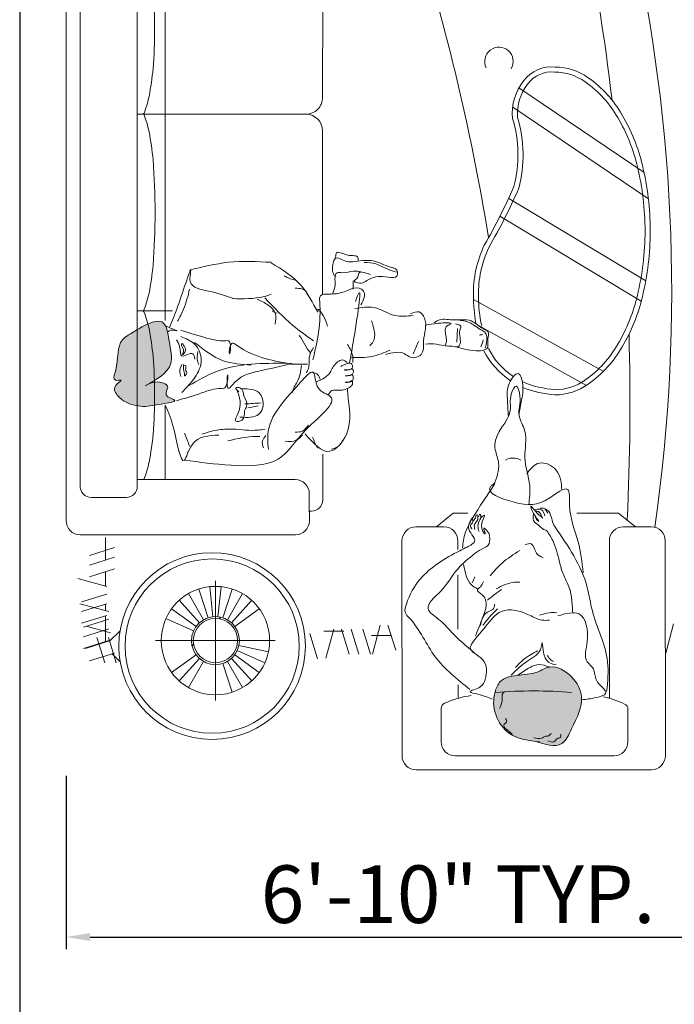
# Model space of a CAD drawing. Units: millimetres. Extents: x 20768 to 23556, y 50760 to 52704.
# Tile 10 of 36: x 20908 to 20976, y 51904 to 52007. Entities that reach past the tile are written whole.
import ezdxf

# ---------------------------------------------------------------- set-up
doc = ezdxf.new("R2010")
doc.units = ezdxf.units.MM
doc.layers.add('A-FURN', color=8, linetype='Continuous', lineweight=18)
doc.layers.add('S-ANNO-DIMS', color=2, linetype='Continuous', lineweight=18)
doc.styles.get("Standard").update_dxf_attribs({"font": 'arial.ttf'})
doc.dimstyles.new('ISO-25', dxfattribs={"dimtxt": 6, "dimasz": 2.5, "dimexe": 1.25, "dimexo": 0.625, "dimtad": 1, "dimdec": 0, "dimlunit": 3, "dimtxsty": 'Standard', "dimcen": 2.5, "dimadec": 0, "dimazin": 0, "dimtfac": 1, "dimtdec": 0, "dimtmove": 0, "dimatfit": 3, "dimfxl": 1, "dimarcsym": 0})

# ---------------------------------------------------------------- blocks, each defined once
blk = doc.blocks.new('A$C32DD204E')
at = {"ltscale": 3}
h = blk.add_hatch(color=256, dxfattribs=at)
edge = h.paths.add_edge_path()
edge.add_spline(control_points=[(248.5, 1171), (279.6, 1188.5), (331.5, 1220.4), (312.1, 1296.2), (303.9, 1374.7), (243.4, 1354.4), (209.2, 1331.9), (147.9, 1299.6), (163.4, 1244.6), (138.6, 1178), (180.2, 1188.1), (136, 1164), (157.4, 1133.7), (185.5, 1110.9), (241.5, 1099.6), (276.6, 1109.9), (350.3, 1120.6), (292.2, 1133.5), (320.4, 1170.6), (274.8, 1182.2), (255.2, 1174.5), (248.5, 1171)], knot_values=[6.92976, 6.92976, 6.92976, 6.92976, 88.633957, 150.80248, 204.81141, 248.139794, 279.389018, 321.893636, 408.375761, 431.643524, 447.144857, 469.07466, 497.305108, 522.125936, 570.063074, 628.708388, 656.922664, 684.873946, 704.64736, 740.083308, 760.727208, 760.727208, 760.727208, 760.727208], degree=3, periodic=0)
h = blk.add_hatch(color=256, dxfattribs=at)
edge = h.paths.add_edge_path()
edge.add_spline(control_points=[(1426.4, 86.6), (1397.7, 90.1), (1345.7, 99.1), (1298.9, 165.8), (1296.3, 225.7), (1328.2, 297.6), (1410.2, 279.3), (1477.3, 324.4), (1540.8, 288.1), (1580.5, 210.8), (1543, 141.8), (1506.8, 60.6), (1456.5, 76.7), (1426.4, 86.6)], knot_values=[11.171972, 11.171972, 11.171972, 11.171972, 83.935274, 146.390702, 207.043537, 236.474222, 338.687878, 374.142978, 438.985032, 497.846364, 587.349285, 634.808067, 704.959464, 704.959464, 704.959464, 704.959464], degree=3, periodic=0)
for p, q in [((0, 755.3, -685.7), (0.2, 2629.6, -685.7)), ((779.4, 2042.5, -685.7), (779.6, 2565.6, -685.7)), ((42.1, 861.2, -685.7), (42.7, 2524.3, -685.7)), ((216, 1393.9, -685.7), (216.2, 2524.2, -685.7)), ((301, 1394, -685.7), (301.2, 2504.1, -685.7)), ((1375.8, 2071.1, -685.7), (1756.4, 1813.8, -685.7)), ((1356.9, 2013.1, -685.7), (1769.1, 1734.5, -685.7)), ((216, 1991.7, -685.7), (595.7, 1991.5, -685.7)), ((595.7, 1991.5, -685.7), (728.3, 1991.5, -685.7)), ((779.4, 1940.4, -685.7), (779.4, 1445.2, -685.7)), ((1345.3, 1735.8, -685.7), (1761.4, 1485.6, -685.7)), ((1318.2, 1681.4, -685.7), (1747.5, 1423.2, -685.7)), ((1237.5, 1428.9, -685.7), (1632.1, 1210.6, -685.7)), ((216, 1394.2, -685.7), (216.2, 861.4, -685.7)), ((216, 1393.9, -685.7), (323, 1394, -685.7)), ((301, 1394.2, -685.7), (301, 1364.8, -685.7)), ((1245.7, 1353.6, -685.7), (1581.4, 1167.9, -685.7)), ((1188.7, 1340.5), (1187.5, 1298.8)), ((301.1, 1106.9, -685.7), (301.2, 881.5, -685.7)), ((370.5, 964.2), (368.9, 965.7)), ((779.5, 959.1, -685.7), (779.6, 820, -685.7)), ((216.2, 881.5, -685.7), (696.3, 881.7, -685.7)), ((738.8, 782.8, -685.7), (738.8, 839.2, -685.7)), ((76.8, 827.3, -685.7), (182.2, 827.3, -685.7)), ((739.1, 787, -685.7), (739.1, 756.3, -685.7)), ((739.1, 785.9, -685.7), (745.6, 785.9, -685.7)), ((1125.7, 738.2, -685.7), (1176, 779.7, -685.7)), ((1220.3, 779.7, -685.7), (1176, 779.7, -685.7)), ((1678.7, 779.9, -685.7), (1551.9, 779.9, -685.7)), ((1729.9, 737.7, -685.7), (1678.7, 779.9, -685.7)), ((1148, 738.2, -685.7), (1062.9, 738.1, -685.7)), ((1778.1, 738.4, -685.7), (1693.1, 738.4, -685.7)), ((42.8, 713.5, -685.7), (696.6, 713.7, -685.7)), ((1020.4, 695.6, -685.7), (1020.7, 42.5, -685.7)), ((1190.5, 669.7, -685.7), (1190.5, 695.7, -685.7)), ((1650.7, 217.2, -685.7), (1650.6, 695.8, -685.7)), ((1820.9, 42.8, -685.7), (1820.7, 695.9, -685.7)), ((147, 675, -685.7), (70.5, 651.5, -685.7)), ((147, 645.6, -685.7), (70.5, 622.1, -685.7)), ((147, 610.3, -685.7), (70.5, 586.8, -685.7)), ((123.5, 557.3, -685.7), (35.3, 580.9, -685.7)), ((453.6, 392.6, -685.7), (453.6, 574.3, -685.7)), ((1190.6, 427.1, -685.7), (1190.6, 592.2, -685.7)), ((431.1, 461.8, -685.7), (402.7, 549.2, -685.7)), ((446, 465, -685.7), (436.4, 556.4, -685.7)), ((461.2, 465, -685.7), (470.8, 556.4, -685.7)), ((476.1, 461.8, -685.7), (504.5, 549.2, -685.7)), ((123.5, 533.8, -685.7), (47, 510.3, -685.7)), ((404.9, 446.7, -685.7), (343.4, 515, -685.7)), ((417.2, 455.6, -685.7), (371.3, 535.2, -685.7)), ((490, 455.6, -685.7), (536, 535.2, -685.7)), ((502.3, 446.7, -685.7), (563.8, 515, -685.7)), ((129.3, 480.9, -685.7), (41.1, 504.4, -685.7)), ((123.5, 504.4, -685.7), (47, 480.9, -685.7)), ((394.8, 435.4, -685.7), (320.4, 489.4, -685.7)), ((512.5, 435.4, -685.7), (586.9, 489.4, -685.7)), ((123.5, 469.1, -685.7), (47, 445.6, -685.7)), ((129.3, 457.3, -685.7), (52.9, 433.8, -685.7)), ((387.1, 422.2, -685.7), (303.2, 459.6, -685.7)), ((469.9, 463.5, -685.7), (465.2, 458.8, -685.7)), ((129.3, 427.9, -685.7), (52.9, 404.4, -685.7)), ((135.2, 416.2, -685.7), (60.4, 436.1, -685.7)), ((163.9, 422.7, -685.7), (132.1, 390.9, -685.7)), ((783.1, 421.6), (843.8, 421.6)), ((813.1, 427.8, -685.7), (789.5, 339.6, -685.7)), ((836.6, 427.8, -685.7), (860.1, 351.4, -685.7)), ((866, 427.8, -685.7), (889.5, 351.4, -685.7)), ((901.3, 427.8, -685.7), (924.8, 351.4, -685.7)), ((954.3, 439.6, -685.7), (930.7, 351.4, -685.7)), ((977.8, 439.6, -685.7), (1001.3, 363.1, -685.7)), ((1822.4, 354.9, -685.7), (1846, 443.1, -685.7)), ((129.3, 392.6, -685.7), (52.9, 369.1, -685.7)), ((135.2, 392.6, -685.7), (58.8, 369.1, -685.7)), ((117, 325.5, -685.7), (93.5, 401.9, -685.7)), ((152.3, 325.5, -685.7), (128.8, 401.9, -685.7)), ((453.6, 392.6, -685.7), (271.9, 392.6, -685.7)), ((453.6, 392.6, -685.7), (453.6, 210.9, -685.7)), ((453.6, 392.6, -685.7), (635.4, 392.6, -685.7)), ((764.1, 337.3, -685.7), (740.6, 413.7, -685.7)), ((928.1, 408.1), (988.8, 408.1)), ((387.4, 381, -685.7), (382.7, 376.3, -685.7)), ((520.1, 363, -685.7), (604.1, 325.6, -685.7)), ((524.8, 377.5, -685.7), (614.7, 358.3, -685.7)), ((147, 354.5, -685.7), (70.5, 331, -685.7)), ((139.9, 352.3, -685.7), (164.1, 328, -685.7)), ((394.8, 349.8, -685.7), (320.4, 295.8, -685.7)), ((404.9, 338.5, -685.7), (343.4, 270.2, -685.7)), ((417.2, 329.6, -685.7), (371.3, 249.9, -685.7)), ((490, 329.6, -685.7), (536, 249.9, -685.7)), ((502.3, 338.5, -685.7), (563.8, 270.2, -685.7)), ((512.5, 349.8, -685.7), (586.9, 295.8, -685.7)), ((476.1, 323.4, -685.7), (504.5, 235.9, -685.7)), ((1190.7, 217.1, -685.7), (1190.7, 258.6, -685.7)), ((1139.7, 85.1, -685.7), (1139.7, 186.8, -685.7)), ((1707.1, 85.3, -685.7), (1707, 184.5, -685.7)), ((1182.2, 42.6, -685.7), (1664.6, 42.8, -685.7)), ((1063.2, 0, -685.7), (1778.4, 0.3, -685.7))]:
    blk.add_line(p, q)
at = {"elevation": -685.7}
for points in [[(268.9, 2248, 0.02107), (264, 2366.2, 0.029233), (251.9, 2450.6, 0.045778), (235.8, 2504.1, 0.201615)], [(234.8, 1392.4, 0.047423), (251.7, 1447.7, 0.029233), (263.9, 1532.1, 0.017749), (270.5, 1692.8, 0.02107)], [(234.8, 1395.5, -0.047423), (251.7, 1340.2, -0.029233), (263.9, 1255.7, -0.02107), (268.9, 1137.6, -0.02107)], [(236, 1394.2, -0.00246), (234.8, 1391.4)], [(268.9, 1137.6, -0.02107), (264, 1019.4, -0.029233), (251.9, 935, -0.045778), (235.8, 881.5, -0.201615)]]:
    blk.add_lwpolyline(points, format="xyb", dxfattribs=at)
for points in [[(119.4, 705.9), (119.4, 637.1)], [(119.4, 601.8), (119.4, 558.4)], [(119.4, 503.2), (119.4, 483.5)], [(119.4, 467.9), (119.4, 387.8)]]:
    blk.add_lwpolyline(points, dxfattribs=at)
for centre, radius in [((443.5, 376, -685.7), 283.5), ((443.5, 376, -685.7), 264.6), ((453.6, 392.6, -685.7), 164.7), ((453.6, 392.6, -685.7), 72.8), ((453.6, 392.6, -685.7), 67.2)]:
    blk.add_circle(centre, radius)
for centre, radius, start, end in [((-5717.4, 460.8, -685.7), 7095.9, 9.37507, 17.5955), ((-6034.3, 1118.6, -685.7), 7747.5, 6.78419, 11.06631), ((-3160.4, 1453.5, -685.7), 5000.5, 351.7639, 13.5399), ((-1135.1, 2248.6, -685.7), 1404, 355.1489, 359.9772), ((1315, 2151.6, -685.7), 43.3, 329.4196, 206.4089), ((-463.5, 2191.6, -685.7), 730, 348.451, 355.1489), ((1474.3, 2030.8, -685.7), 104.3, 83.9251, 143.2199), ((1485.3, 1960, -685.7), 174.6, 54.5394, 90), ((1474.3, 2030.8, -685.7), 88.8, 83.3999, 143.3893), ((1485.3, 1960, -685.7), 159, 54.5394, 90.3034), ((1375.6, 1805.9, -685.7), 363.7, 30.1802, 54.5394), ((1514.9, 1993.6, -685.7), 159.2, 141.263, 185.4473), ((1514.9, 1993.6, -685.7), 143.6, 141.1552, 184.8436), ((1375.6, 1805.9, -685.7), 348.1, 30.1802, 54.5394), ((-47.7, 2106.6, -685.7), 305.7, 337.5906, 348.451), ((728.3, 2042.5, -685.7), 51, 269.9772, 359.9772), ((-47.8, 1877.9, -685.7), 305.7, 21.7999, 22.3637), ((-47.7, 1876.7, -685.7), 305.7, 11.549, 22.4094), ((728.3, 1940.4, -685.7), 51, 0.0228, 90.0228), ((993.4, 1867.9, -685.7), 379.5, 345.261, 16.9432), ((993.4, 1867.9, -685.7), 395.1, 345.0883, 16.7074), ((1200.1, 1703.8, -685.7), 551.1, 13.5438, 30.1802), ((1200.1, 1703.8, -685.7), 566.7, 13.5438, 30.1802), ((-463.5, 1791.7, -685.7), 730, 4.8511, 11.549), ((-1995, 1680, -685.7), 2265.5, 0.3248, 4.3921), ((921.7, 1636.8, -685.7), 837.4, 0, 13.5438), ((921.7, 1636.8, -685.7), 853, 0, 13.5438), ((-174.4, 2435.8, -685.7), 1672.4, 329.7762, 336.5922), ((-174.4, 2435.8, -685.7), 1688, 329.7992, 336.632), ((921.7, 1636.8, -685.7), 837.4, 346.4562, 0), ((921.7, 1636.8, -685.7), 853, 346.4562, 0), ((1584.9, 1445.2, -685.7), 347.6, 154.6827, 181.0708), ((1584.9, 1445.2, -685.7), 332, 154.7964, 181.089), ((1699.8, 1441.1, -685.7), 462.4, 180.2965, 190.3289), ((1699.8, 1441.1, -685.7), 446.9, 180.283, 192.0106), ((1200.1, 1569.7, -685.7), 551.1, 329.8198, 346.4562), ((1200.1, 1569.7, -685.7), 566.7, 329.8198, 346.4562), ((464.9, -539.7), 1961.2, 81.0036, 81.3607), ((631.8, -596.5), 1995.1, 85.9802, 86.2563), ((-6034.3, 1118.6, -685.7), 7747.5, 357.33463, 1.51542), ((1375.6, 1467.7, -685.7), 348.1, 305.4606, 329.8198), ((1486, 1384.5, -685.7), 244, 207.1509, 235.8302), ((1486, 1384.5, -685.7), 228.4, 207.3492, 235.7987), ((1375.6, 1467.7, -685.7), 363.7, 305.4606, 329.8198), ((1509.1, 1466.2, -685.7), 312.4, 247.051, 265.7344), ((1485.3, 1313.6, -685.7), 174.6, 270, 305.4606), ((1485.3, 1313.6, -685.7), 159, 270.2019, 305.4606), ((1509.1, 1466.2, -685.7), 328, 248.6473, 265.8394), ((696.3, 839.1, -685.7), 42.5, 0.0228, 90.0228), ((77.2, 862.5, -685.7), 35.2, 177.8872, 269.238), ((182.2, 861.4, -685.7), 34, 270.0228, 0.0228), ((745.5, 820, -685.7), 34, 270.0228, 0.0228), ((42.9, 756.4, -685.7), 42.9, 178.4457, 269.7882), ((696.5, 756.3, -685.7), 42.5, 270.0228, 0.0228), ((1063, 695.6, -685.7), 42.5, 90.0228, 180.0228), ((1148, 695.6, -685.7), 42.5, 0.0228, 90.0228), ((1693.1, 695.9, -685.7), 42.5, 90.0228, 180.0228), ((1778.1, 695.9, -685.7), 42.5, 0.0228, 90.0228), ((1421.2, -1279.2, -685.7), 1518.9, 90.0228, 94.419), ((1421.2, -1279.2, -685.7), 1518.9, 85.6266, 90.0228), ((1280.5, -94.8, -685.7), 324.6, 100.5374, 113.7374), ((1364.6, -547, -685.7), 784.5, 99.8363, 100.5374), ((1560.9, -94.7, -685.7), 324.6, 65.1817, 77.2735), ((1156.7, 186.8, -685.7), 17, 113.7374, 180.0228), ((1690, 184.5, -685.7), 17, 0.0228, 65.1817), ((1182.2, 85.1, -685.7), 42.5, 180.0228, 270.0228), ((1664.6, 85.3, -685.7), 42.5, 270.0228, 0.0228), ((1063.2, 42.5, -685.7), 42.5, 180.0228, 270.0228), ((1778.4, 42.8, -685.7), 42.5, 270.0228, 0.0228)]:
    blk.add_arc(centre, radius, start, end)
at = {"ltscale": 3}
for centre, radius, start, end in [((1357, 906.6), 40.6, 79.5148, 123.0894), ((1352, 880), 67.7, 63.6392, 79.5148)]:
    blk.add_arc(centre, radius, start, end, dxfattribs=at)
for points, knots in [([(815.6, 1499.7), (813.2, 1505.1), (807.5, 1517.9), (809.7, 1535.9), (818.3, 1563.8), (849.5, 1539.3), (888.8, 1546.3), (939.9, 1551.3), (976, 1527), (1006.1, 1522.5), (1011, 1491), (964.4, 1500), (925.8, 1499.2), (898.4, 1471.9), (869.3, 1485.1), (891, 1492.1), (886, 1512.2), (894.6, 1511.6), (895.6, 1511.5)], [0, 0, 0, 0, 15.214729, 36.055512, 48.857472, 79.738512, 103.122769, 157.685733, 206.194273, 214.411126, 234.296897, 257.825245, 307.464974, 341.56748, 352.042995, 362.192251, 380.803332, 383.401633, 383.401633, 383.401633, 383.401633]), ([(817.1, 1553), (818.2, 1556.2), (819.7, 1561), (820, 1579.5), (854.5, 1556.5), (888.8, 1565.3), (887.1, 1549.5), (886.7, 1545.6)], [0, 0, 0, 0, 9.109215, 13.285838, 44.707752, 72.752889, 81.852859, 81.852859, 81.852859, 81.852859]), ([(314.5, 1345.5), (321.9, 1362.7), (341.1, 1407.4), (387.3, 1556.5), (369.3, 1464.2), (445.2, 1454.4), (487.7, 1439.1), (511.9, 1430.4)], [0, 0, 0, 0, 60.518576, 156.742964, 182.299185, 237.275016, 309.902587, 309.902587, 309.902587, 309.902587]), ([(374.5, 1517.7), (413.9, 1527.5), (495.5, 1547.9), (579.6, 1543.7), (622.9, 1541.5)], [0, 0, 0, 0, 106.409885, 220.025525, 220.025525, 220.025525, 220.025525]), ([(623, 1540.2), (656.5, 1519.3), (716.8, 1481.5), (749.4, 1418.6), (764, 1390.6)], [0, 0, 0, 0, 101.553402, 183.196527, 183.196527, 183.196527, 183.196527]), ([(906, 1541.1), (918.1, 1540.7), (943.5, 1539.6), (973.1, 1520.3), (994.7, 1514.1), (1003.7, 1511.5)], [0, 0, 0, 0, 31.421868, 65.723795, 90.374568, 90.374568, 90.374568, 90.374568]), ([(662.7, 1500.2), (666.7, 1498), (679.3, 1491.4), (693.1, 1487.5), (702.4, 1484.9)], [0, 0, 0, 0, 12.001288, 37.458402, 37.458402, 37.458402, 37.458402]), ([(809.7, 1446.3), (813.1, 1455.2), (819.4, 1471.8), (815.4, 1492.1), (820.4, 1513), (846.6, 1507.3), (878.7, 1519.8), (907.7, 1510), (925.2, 1504.1)], [0, 0, 0, 0, 24.284632, 45.084884, 56.190964, 71.83444, 101.967681, 148.338712, 148.338712, 148.338712, 148.338712]), ([(895.2, 1411.9), (903.3, 1427.4), (912.7, 1445.6), (880, 1477.1), (837.9, 1433.9), (767.6, 1451.2), (776.7, 1361.9), (762.8, 1301.5), (749.8, 1245.2)], [0, 0, 0, 0, 37.77004, 44.330448, 112.206702, 158.127425, 169.373671, 326.046663, 326.046663, 326.046663, 326.046663]), ([(861.3, 1235.3), (864.2, 1253), (878.2, 1331.2), (903.8, 1491.5), (882.2, 1430.6), (879.3, 1422.5)], [229.252261, 229.252261, 229.252261, 229.252261, 259.312026, 344.867622, 358.082672, 358.082672, 358.082672, 358.082672]), ([(871.9, 1484.8), (871.9, 1477.9), (871.9, 1469.5), (871.9, 1461.1), (871.9, 1459.6)], [0, 0, 0, 0, 18.199941, 22.100035, 22.100035, 22.100035, 22.100035]), ([(338.4, 1362.4), (345, 1374.5), (361.7, 1405.4), (370, 1439.6), (375.1, 1460.4)], [0, 0, 0, 0, 36.019014, 92.081432, 92.081432, 92.081432, 92.081432]), ([(505.6, 1431.2), (538.2, 1430.5), (578.2, 1429.6), (616, 1441.7), (623, 1444)], [0, 0, 0, 0, 84.476355, 104.032988, 104.032988, 104.032988, 104.032988]), ([(696.3, 1463.4), (710.4, 1462.2), (728.4, 1460.6), (732.2, 1445.3), (733, 1442)], [0, 0, 0, 0, 31.408902, 39.899476, 39.899476, 39.899476, 39.899476]), ([(580.1, 1429.8), (591.5, 1424.4), (612.6, 1414.6), (640.6, 1388.2), (637, 1365), (635.1, 1353.2)], [0, 0, 0, 0, 33.626167, 62.160116, 91.695701, 91.695701, 91.695701, 91.695701]), ([(603.8, 1433.3), (631.3, 1404.4), (676.7, 1356.7), (730.1, 1318.2), (751.2, 1303)], [0, 0, 0, 0, 104.676597, 172.875133, 172.875133, 172.875133, 172.875133]), ([(877.4, 1401.3), (897.1, 1404.5), (939.9, 1411.6), (993.7, 1373.5), (1035.6, 1378.1), (1054.5, 1380.1)], [0, 0, 0, 0, 51.063738, 110.501338, 159.193788, 159.193788, 159.193788, 159.193788]), ([(772.8, 1393), (778.4, 1384.1), (787.5, 1369.7), (792.4, 1353.3), (794.2, 1347.1)], [0, 0, 0, 0, 27.640179, 44.620551, 44.620551, 44.620551, 44.620551]), ([(969.9, 1261.1), (990.7, 1266.8), (1019.1, 1274.6), (1048.1, 1247.4), (1089.5, 1258.3), (1081.3, 1314.7), (1101.6, 1357.4), (1073.7, 1397.1), (1055.9, 1389.4), (1046.5, 1385.4)], [0, 0, 0, 0, 51.063966, 69.760857, 98.442485, 136.21289, 196.583877, 217.96974, 241.616381, 241.616381, 241.616381, 241.616381]), ([(240.5, 1166.5), (274.5, 1185.5), (332.2, 1217.8), (312.1, 1296.2), (303.9, 1374.7), (243.4, 1354.4), (209.2, 1331.9), (147.9, 1299.6), (163.4, 1244.6), (138.6, 1178), (180.2, 1188.1), (136, 1164), (157.4, 1133.7), (185.5, 1110.9), (241.5, 1099.6), (276.6, 1109.9), (350.3, 1120.6), (292.2, 1133.5), (320.4, 1170.6), (269.8, 1183.5), (249.6, 1171.8), (240.5, 1166.5)], [0, 0, 0, 0, 88.633957, 150.80248, 204.81141, 248.139794, 279.389018, 321.893636, 408.375761, 431.643524, 447.144857, 469.07466, 497.305108, 522.125936, 570.063074, 628.708388, 656.922664, 684.873946, 704.64736, 740.083308, 769.084366, 769.084366, 769.084366, 769.084366]), ([(309.6, 1329.3), (310.5, 1331), (315, 1339.5), (351.8, 1328.4), (322, 1340.1), (304, 1347.2)], [0, 0, 0, 0, 4.957486, 24.33421, 53.851131, 53.851131, 53.851131, 53.851131]), ([(927.6, 1364.2), (935.3, 1341.3), (945, 1312.2), (926.2, 1291.8), (922.3, 1287.5)], [0, 0, 0, 0, 55.878701, 70.732003, 70.732003, 70.732003, 70.732003]), ([(1094.1, 1351), (1103.8, 1352.9), (1123.3, 1356.8), (1183.4, 1359.1), (1146, 1345.7), (1156.4, 1319.3), (1156, 1283.3), (1121, 1296.3), (1102.2, 1294.1), (1091.5, 1292.8)], [0, 0, 0, 0, 32.791493, 65.856029, 77.112898, 107.365096, 127.973901, 150.397914, 180.540849, 180.540849, 180.540849, 180.540849]), ([(1118, 1358.2), (1121.8, 1360.9), (1138, 1372), (1178.1, 1363), (1230.2, 1373), (1257, 1342.7), (1288.6, 1331.3), (1278.1, 1306), (1286.4, 1273), (1223.1, 1270.5), (1188.8, 1286.7), (1158.9, 1287.5), (1151.8, 1287.7)], [0, 0, 0, 0, 12.05449, 50.662285, 100.751119, 139.349436, 152.871984, 178.39508, 194.636814, 232.879132, 291.995735, 310.219291, 310.219291, 310.219291, 310.219291]), ([(1183.4, 1354.2), (1190.9, 1352.9), (1203.6, 1350.5), (1189.2, 1323.8), (1204.2, 1303.5), (1191.8, 1283.5), (1185.8, 1284.4), (1183.1, 1284.9)], [0, 0, 0, 0, 15.405528, 26.125312, 63.82535, 72.147315, 78.642841, 78.642841, 78.642841, 78.642841]), ([(1190.6, 1366.4), (1202.4, 1365), (1228.5, 1361.8), (1250.9, 1340.1), (1273.6, 1330.7), (1281.3, 1309.2), (1276.7, 1293.2), (1273.5, 1281.9)], [0, 0, 0, 0, 30.578618, 67.353333, 79.611572, 92.413964, 122.566762, 122.566762, 122.566762, 122.566762]), ([(348, 1335.2), (378.1, 1325.8), (423.4, 1311.5), (470.9, 1300.8), (505.7, 1306.7), (492.8, 1231.6), (496.4, 1304.6), (545.6, 1270.4), (599.6, 1246.5), (663.3, 1236.7), (694.3, 1232)], [0, 0, 0, 0, 82.179012, 124.172551, 131.128421, 166.009294, 194.708047, 207.195703, 291.828264, 372.00922, 372.00922, 372.00922, 372.00922]), ([(348.4, 1315.8), (363.7, 1309.9), (395.9, 1297.5), (418.6, 1242), (392.1, 1188.2), (365.5, 1160.4), (351.7, 1146)], [0, 0, 0, 0, 41.941762, 88.289003, 137.229401, 190.028503, 190.028503, 190.028503, 190.028503]), ([(335.3, 1306), (339.3, 1299.3), (347.7, 1285.3), (345.8, 1247.6), (369.4, 1263.9), (388.2, 1265.3), (389.8, 1254.3), (390.8, 1247.2)], [0, 0, 0, 0, 21.811235, 45.429417, 66.268319, 74.855405, 90.278481, 90.278481, 90.278481, 90.278481]), ([(350.6, 1295.1), (350.5, 1293), (349.7, 1284.3), (361.3, 1275.9), (349.4, 1255.1), (369.1, 1276.1), (357.7, 1286), (354.6, 1293), (353.7, 1295.1)], [0, 0, 0, 0, 5.37014, 22.350864, 30.841366, 44.263375, 58.721741, 64.724876, 64.724876, 64.724876, 64.724876]), ([(390.3, 1298.1), (418.1, 1276), (468.7, 1235.6), (533, 1231.3), (562.2, 1229.4)], [0, 0, 0, 0, 90.713488, 165.812862, 165.812862, 165.812862, 165.812862]), ([(855.4, 1292), (862.2, 1280.1), (872.2, 1262.7), (871, 1243.1), (870.7, 1236.9)], [0, 0, 0, 0, 34.902027, 51.012448, 51.012448, 51.012448, 51.012448]), ([(399.6, 1270.6), (398.4, 1260.2), (396.8, 1246.5), (401.5, 1233.8), (402.6, 1230.8)], [0, 0, 0, 0, 26.8507, 35.340922, 35.340922, 35.340922, 35.340922]), ([(751.4, 1282.8), (746.1, 1274), (734.5, 1254.2), (741, 1225.1), (732.3, 1210.3), (730, 1206.3)], [0, 0, 0, 0, 26.441749, 58.774114, 70.780485, 70.780485, 70.780485, 70.780485]), ([(864.1, 1253.2), (886.5, 1252.3), (927.8, 1250.7), (965.7, 1266.9), (983.1, 1274.3)], [0, 0, 0, 0, 58.013512, 107.149157, 107.149157, 107.149157, 107.149157]), ([(334.8, 1120.9), (360.4, 1128.3), (405.8, 1141.5), (452.6, 1160.2), (491.3, 1155.9), (493, 1241.6), (484.9, 1142.7), (524.3, 1197.5), (588.2, 1210.9), (652.5, 1226.4), (686.4, 1234.7)], [0, 0, 0, 0, 70.409867, 124.986685, 129.624235, 168.516696, 205.713361, 218.8346, 299.734666, 390.28545, 390.28545, 390.28545, 390.28545]), ([(351.7, 1230.9), (348.5, 1224.4), (342.8, 1212.8), (346.7, 1200.5), (348.4, 1195)], [0, 0, 0, 0, 18.113831, 32.718438, 32.718438, 32.718438, 32.718438]), ([(356.8, 1230.8), (356.3, 1225.5), (355.3, 1214.9), (360.7, 1205.6), (359.1, 1194), (370.8, 1206.3), (359, 1213.3), (366.7, 1228.5), (361, 1227.9), (359.8, 1227.7)], [0, 0, 0, 0, 13.425536, 27.116244, 29.801129, 37.393081, 48.463136, 59.203416, 61.886553, 61.886553, 61.886553, 61.886553]), ([(371.8, 1165.9), (400.4, 1182.7), (490.8, 1235.8), (597.5, 1235.1), (670.5, 1234.7)], [0, 0, 0, 0, 86.085059, 272.751702, 272.751702, 272.751702, 272.751702]), ([(714.7, 1227.7), (712.6, 1210.6), (709.9, 1187.3), (691.9, 1163.5), (688.8, 1151.4), (687.1, 1145.1)], [0, 0, 0, 0, 44.281186, 59.934993, 76.915365, 76.915365, 76.915365, 76.915365]), ([(760.7, 1178.5), (777.8, 1186), (795.8, 1193.8), (808.8, 1220.7), (817.6, 1235.9), (839.6, 1248.1), (848.9, 1241.2), (853.6, 1237.7)], [0, 0, 0, 0, 45.537019, 47.905206, 78.191519, 91.952902, 106.155728, 106.155728, 106.155728, 106.155728]), ([(796.9, 1139.9), (800.1, 1144.8), (807.4, 1155.9), (834.8, 1150.8), (858.6, 1157), (872.2, 1171.5), (868.5, 1186.6), (860.5, 1174.8), (843.8, 1177.9), (862.3, 1176.4), (874.3, 1181.8), (871.9, 1204.3), (860, 1196.4), (840.8, 1196.3), (860.8, 1197.9), (873.3, 1198.7), (874, 1221), (859.5, 1214.2), (834.1, 1215.5), (865.4, 1212.3), (872.4, 1225.4), (866.1, 1236.7), (854.1, 1234.8), (844.5, 1230), (838, 1227.2), (834.3, 1225.6)], [0, 0, 0, 0, 14.245589, 32.27085, 65.424938, 75.415665, 83.125969, 92.594533, 101.062211, 108.471373, 123.178778, 136.06387, 144.792436, 155.430033, 166.067631, 176.109786, 189.879186, 198.412834, 212.213818, 230.332194, 238.870274, 247.408355, 257.993066, 266.055047, 276.480967, 276.480967, 276.480967, 276.480967]), ([(359.2, 940.8), (405, 934.5), (496.9, 921.8), (657.2, 922.9), (708.4, 1030.4), (845.8, 1129.3), (754.4, 1150.7), (759.2, 1230.2), (662.8, 1120.6), (605, 1063.1), (613.7, 984.5), (615, 972.8)], [0, 0, 0, 0, 125.422801, 251.68088, 363.259103, 469.510953, 507.917449, 552.801864, 594.966396, 768.088902, 798.341471, 798.341471, 798.341471, 798.341471]), ([(749.9, 1207.5), (755.3, 1205.7), (765.7, 1202.1), (769.7, 1191.9), (771.6, 1186.9)], [0, 0, 0, 0, 14.202992, 27.472435, 27.472435, 27.472435, 27.472435]), ([(1343.7, 1073.5), (1342.6, 1091.5), (1340.7, 1125.6), (1338.5, 1168.8), (1378.1, 1222.7), (1390.8, 1161.5), (1384.6, 1125), (1379.2, 1097.9), (1376.2, 1082.4)], [0, 0, 0, 0, 46.697433, 88.465151, 123.324676, 161.835136, 191.877979, 232.626852, 232.626852, 232.626852, 232.626852]), ([(518.9, 1154.3), (526.9, 1132.1), (537.4, 1103.2), (507.2, 1054.7), (545.6, 1061.6), (538.1, 1089.1), (555, 1112.1), (536.7, 1133.8), (538, 1161.8), (509.4, 1162.3), (519.4, 1153.2), (525, 1148.2)], [0, 0, 0, 0, 64.497154, 84.043581, 100.365205, 128.396624, 142.854646, 168.325592, 192.338234, 203.071238, 216.493247, 216.493247, 216.493247, 216.493247]), ([(534.2, 1157.3), (554.1, 1157.1), (589.5, 1156.6), (603.8, 1109.4), (582.9, 1067.4), (550.3, 1069.9), (528.1, 1071.6)], [0, 0, 0, 0, 46.862522, 83.38104, 107.393682, 159.00759, 159.00759, 159.00759, 159.00759]), ([(726.7, 1020.4), (751.1, 991.9), (795, 940.9), (875.3, 1034.1), (857.4, 1111.5), (854.9, 1152.3), (854.7, 1157.9)], [0, 0, 0, 0, 53.201817, 95.441996, 166.7115, 178.37996, 178.37996, 178.37996, 178.37996]), ([(1299.3, 863.8), (1308, 886.5), (1318.6, 914), (1309.4, 955.4), (1287.5, 1011.9), (1362.9, 1071.8), (1344.1, 1129.9), (1369.3, 1179.2), (1386.1, 1119.1), (1366.1, 1080.1), (1406.2, 1020.5), (1384.3, 946.3), (1413.8, 873.4), (1408.1, 824.6), (1405.7, 804.8)], [0, 0, 0, 0, 60.970115, 74.178445, 111.267097, 210.963126, 255.074467, 279.515708, 307.41666, 359.287359, 403.554034, 473.492101, 549.720465, 601.59141, 601.59141, 601.59141, 601.59141]), ([(300.5, 1107.7), (308.7, 1090.3), (330.5, 1043.9), (351.6, 894), (382, 1013), (432.6, 1015.3), (464.2, 1016.7)], [0, 0, 0, 0, 58.099529, 155.224826, 201.006913, 277.065022, 277.065022, 277.065022, 277.065022]), ([(696.3, 1025.7), (703.9, 1025.8), (720.6, 1026), (730.6, 1039.7), (736.1, 1047.2)], [0, 0, 0, 0, 18.973621, 41.74948, 41.74948, 41.74948, 41.74948]), ([(411.8, 1019.6), (427, 1024.3), (457.8, 1033.9), (515.9, 1036.8), (565, 1028.3), (597.4, 1033.7), (604.5, 1034.9)], [0, 0, 0, 0, 41.657024, 84.672483, 151.807143, 170.780764, 170.780764, 170.780764, 170.780764]), ([(490.8, 999.2), (519.7, 1005.6), (552.1, 1012.8), (585.1, 1012.5), (588.6, 1012.5)], [0, 0, 0, 0, 77.391086, 86.66573, 86.66573, 86.66573, 86.66573]), ([(607.1, 1015.1), (602.5, 1010.1), (592.9, 999.4), (597, 985.4), (599.2, 978.1)], [0, 0, 0, 0, 16.728024, 35.434645, 35.434645, 35.434645, 35.434645]), ([(665.7, 998.2), (677.7, 997.4), (698.1, 996), (712, 1010.5), (717.7, 1016.5)], [0, 0, 0, 0, 29.637545, 50.599936, 50.599936, 50.599936, 50.599936]), ([(806.4, 973.7), (817.2, 977.3), (832.6, 982.5), (838.3, 996.9), (840.1, 1001.2)], [0, 0, 0, 0, 27.630169, 39.636541, 39.636541, 39.636541, 39.636541]), ([(1506.2, 849.1), (1504.6, 871.7), (1501.6, 913.4), (1435.1, 944.4), (1411.3, 913.9), (1399.8, 899.3)], [0, 0, 0, 0, 56.575903, 104.225618, 148.354052, 148.354052, 148.354052, 148.354052]), ([(1204.8, 674.8), (1205.7, 689.1), (1209.7, 751.6), (1334.2, 902.6), (1270.1, 841.7), (1388.3, 800.1), (1443.9, 802.3), (1533.8, 875.3), (1524.6, 770.6), (1559.6, 702.9), (1567.5, 630.9), (1571.2, 598.1)], [0, 0, 0, 0, 42.167956, 184.846032, 188.510605, 261.118314, 357.582537, 412.070511, 453.838275, 554.467695, 638.871943, 638.871943, 638.871943, 638.871943]), ([(1286.8, 709.7), (1285.8, 714.2), (1283.9, 723.2), (1262.2, 742.3), (1280.9, 705.6), (1248.4, 742.3), (1280.4, 780.7), (1262.2, 768.8), (1255.4, 758.3), (1249.3, 741.3), (1253, 729.3), (1254.6, 724)], [0, 0, 0, 0, 13.622009, 27.045047, 42.301032, 59.74223, 94.71225, 98.491569, 110.440566, 128.701216, 142.844466, 142.844466, 142.844466, 142.844466]), ([(1436.7, 754.6), (1431.6, 760.9), (1422.6, 772.2), (1405.8, 809.4), (1424.2, 788.6), (1433.1, 777), (1442.7, 769.2), (1448, 764.8)], [0, 0, 0, 0, 25.892768, 46.183307, 59.392839, 73.451861, 90.844376, 90.844376, 90.844376, 90.844376]), ([(1454.6, 771.5), (1452.3, 779.3), (1448, 793.7), (1433.4, 792), (1426.6, 791.2)], [0, 0, 0, 0, 18.54008, 34.34859, 34.34859, 34.34859, 34.34859]), ([(1446, 765.9), (1444.7, 770.8), (1442.8, 778), (1437.4, 782.8), (1435.6, 784.3)], [0, 0, 0, 0, 12.899473, 18.839157, 18.839157, 18.839157, 18.839157]), ([(1463.3, 780.1), (1459.8, 786.6), (1454.5, 796.5), (1444.2, 795.2), (1440.6, 794.8)], [0, 0, 0, 0, 16.968689, 25.728505, 25.728505, 25.728505, 25.728505]), ([(1484.6, 738.9), (1481.6, 745.2), (1474.5, 760.5), (1471.1, 786), (1456, 792.4), (1450.6, 794.8)], [0, 0, 0, 0, 18.740722, 44.970985, 59.745283, 59.745283, 59.745283, 59.745283]), ([(1218.4, 676.9), (1223.2, 679.4), (1231.2, 683.6), (1246.3, 695.5), (1231.8, 715.6), (1217.1, 738.3), (1228.1, 756.3), (1234.4, 766.5)], [0, 0, 0, 0, 14.897426, 24.638003, 44.249327, 65.81281, 94.158391, 94.158391, 94.158391, 94.158391]), ([(1234.4, 766.5), (1235.6, 760.9), (1237.7, 752), (1226.1, 742.5), (1230.5, 735.3), (1233.1, 731.2)], [0, 0, 0, 0, 13.770952, 22.047872, 32.93541, 32.93541, 32.93541, 32.93541]), ([(1242.2, 729.9), (1240.7, 735.4), (1237.1, 749.3), (1256.2, 758.7), (1246.7, 779), (1243.7, 762.6), (1238.7, 758), (1235.9, 755.4)], [0, 0, 0, 0, 13.81853, 34.349896, 42.048978, 50.626809, 61.603847, 61.603847, 61.603847, 61.603847]), ([(1253.4, 768.2), (1254.3, 772.5), (1256.4, 781.6), (1262.5, 768.1), (1259.2, 764.5), (1258.1, 763.5)], [0, 0, 0, 0, 7.980072, 16.932683, 20.710806, 20.710806, 20.710806, 20.710806]), ([(1460.8, 726.5), (1456.3, 728), (1446.4, 731.4), (1435.3, 745.4), (1416.8, 751.9), (1420.5, 787.5), (1425.8, 764.3), (1431.5, 757.8), (1435, 755.6), (1436.7, 754.6)], [0, 0, 0, 0, 12.228513, 27.193094, 45.006155, 62.152179, 75.922416, 81.425571, 86.507745, 86.507745, 86.507745, 86.507745]), ([(1538.7, 480), (1537.3, 509.7), (1535.6, 546.2), (1511, 589.6), (1497.9, 632.3), (1488.3, 683.6), (1468, 715.2), (1460.8, 726.5)], [0, 0, 0, 0, 76.228588, 93.60718, 130.36676, 193.495034, 228.582316, 228.582316, 228.582316, 228.582316]), ([(1642.3, 238.3), (1645.5, 268.6), (1654.5, 353.3), (1600.2, 452.9), (1580, 600.7), (1525.2, 680), (1484.6, 738.9)], [0, 0, 0, 0, 78.836785, 220.670789, 284.620897, 468.343596, 468.343596, 468.343596, 468.343596]), ([(1243.2, 658), (1251.1, 663.3), (1263.6, 671.9), (1287.9, 682.2), (1287.2, 698.2), (1286.7, 707.6)], [0, 0, 0, 0, 25.616728, 40.995926, 63.070156, 63.070156, 63.070156, 63.070156]), ([(1395, 684.3), (1401.7, 686.3), (1420.5, 691.7), (1423.9, 655.8), (1441.6, 647.6), (1449.3, 644.1)], [0, 0, 0, 0, 15.981012, 44.422669, 65.960047, 65.960047, 65.960047, 65.960047]), ([(1227, 244.5), (1188.4, 275.1), (1111.6, 335.8), (1074.1, 431.6), (1026, 478.1), (1039.6, 525.5), (1080.9, 600), (1159.3, 647.8), (1210.9, 673.2), (1218.4, 676.9)], [0, 0, 0, 0, 126.89883, 252.166699, 268.447012, 291.91585, 367.798424, 497.771558, 519.675303, 519.675303, 519.675303, 519.675303]), ([(1239.4, 356), (1215.5, 376.2), (1176.8, 409), (1138.6, 455.6), (1079.7, 492.7), (1151.6, 548.5), (1181.6, 608.8), (1224, 642.6), (1243.2, 658)], [0, 0, 0, 0, 80.80909, 130.775511, 169.211303, 225.758914, 301.315819, 364.276194, 364.276194, 364.276194, 364.276194]), ([(1288.3, 589.8), (1299.9, 603.2), (1326.1, 633.3), (1360, 654.4), (1378.9, 666.2)], [0, 0, 0, 0, 46.172455, 104.424665, 104.424665, 104.424665, 104.424665]), ([(1250.1, 549.6), (1243.7, 553.3), (1217.4, 568.3), (1212, 600.1), (1207.9, 624)], [0, 0, 0, 0, 19.085058, 77.715078, 77.715078, 77.715078, 77.715078]), ([(1244.1, 406.9), (1251.2, 424.8), (1266.2, 463), (1288.6, 520.9), (1244, 544.7), (1258.1, 554.6), (1263.8, 562.3), (1266.9, 569), (1268.2, 571.8)], [0, 0, 0, 0, 53.059535, 113.04795, 131.800676, 139.285566, 150.580969, 158.469393, 158.469393, 158.469393, 158.469393]), ([(1306.4, 549.6), (1324.8, 559), (1348, 570.8), (1373.5, 569.9), (1378.9, 569.7)], [0, 0, 0, 0, 52.46729, 66.585747, 66.585747, 66.585747, 66.585747]), ([(1280.3, 515.5), (1289.6, 523), (1303.3, 534.1), (1317.8, 544.3), (1322.5, 547.6)], [0, 0, 0, 0, 31.413427, 46.591217, 46.591217, 46.591217, 46.591217]), ([(1294.9, 214.9), (1282.5, 219.9), (1263.8, 227.4), (1212.6, 238), (1263.1, 248.2), (1278.2, 283.6), (1282, 339.3), (1216.7, 361.1), (1246.3, 402.8), (1275.8, 435), (1322.2, 499.3), (1396.2, 478.5), (1439.4, 452.7), (1460.7, 454.2), (1468.4, 454.7)], [0, 0, 0, 0, 40.880348, 61.700866, 91.143691, 114.873082, 167.923204, 214.466852, 232.950995, 283.095365, 341.741032, 417.680752, 453.135852, 472.889302, 472.889302, 472.889302, 472.889302]), ([(1258.2, 437.1), (1262.1, 454.5), (1267.6, 478.5), (1299, 484.6), (1301.3, 497.2), (1302.4, 503.4)], [0, 0, 0, 0, 41.814842, 57.597678, 72.667081, 72.667081, 72.667081, 72.667081]), ([(1266.2, 439.1), (1274, 449.4), (1287.4, 467.3), (1303.6, 482.8), (1310.5, 489.3)], [0, 0, 0, 0, 33.886621, 58.836239, 58.836239, 58.836239, 58.836239]), ([(1566.7, 212.7), (1580.3, 214.2), (1603.1, 216.8), (1658.3, 232.4), (1602.5, 266.7), (1609, 306.7), (1568.6, 334.3), (1592.3, 396.6), (1575, 491.6), (1518, 474.7), (1493.6, 467.5)], [0, 0, 0, 0, 39.625932, 66.399645, 109.367011, 140.345835, 165.401676, 219.739472, 296.252236, 353.603905, 353.603905, 353.603905, 353.603905]), ([(1438.4, 469.7), (1448.3, 472.9), (1465.4, 478.5), (1483.4, 477.6), (1490.9, 477.2)], [0, 0, 0, 0, 27.147531, 46.900981, 46.900981, 46.900981, 46.900981]), ([(1352.2, 287.8), (1367.9, 303.4), (1397.4, 332.7), (1442.8, 352.2), (1447.6, 404.5), (1446.7, 328.3), (1475.7, 321.8), (1489.2, 318.9)], [0, 0, 0, 0, 58.393088, 109.526114, 121.740606, 162.697201, 197.973392, 197.973392, 197.973392, 197.973392]), ([(1365.9, 310.7), (1373.9, 319.6), (1392.9, 340.5), (1417.9, 353.5), (1432.3, 361.1)], [0, 0, 0, 0, 31.248067, 73.627741, 73.627741, 73.627741, 73.627741]), ([(1480.5, 329), (1475.4, 332.5), (1468.1, 337.5), (1463.6, 345), (1462.1, 347.3)], [0, 0, 0, 0, 15.689416, 22.930946, 22.930946, 22.930946, 22.930946]), ([(1439.7, 85.1), (1406.4, 88.8), (1348.3, 95.3), (1298.9, 165.8), (1296.3, 225.7), (1328.2, 297.6), (1410.2, 279.3), (1477.3, 324.4), (1540.8, 288.1), (1580.5, 210.8), (1543, 141.8), (1506.6, 60.3), (1455.8, 77), (1425.3, 87)], [0, 0, 0, 0, 83.935274, 146.390702, 207.043537, 236.474222, 338.687878, 374.142978, 438.985032, 497.846364, 587.349285, 634.808067, 705.826625, 705.826625, 705.826625, 705.826625]), ([(1372.8, 287.8), (1384.7, 296.2), (1404.3, 309.9), (1438.1, 323.7), (1457.5, 316.4), (1467.8, 312.5)], [0, 0, 0, 0, 38.642267, 63.395223, 91.234873, 91.234873, 91.234873, 91.234873]), ([(1317.1, 186.4), (1320.7, 194.2), (1327.6, 209.1), (1322.2, 229.9), (1331.5, 237.2), (1334.4, 237), (1335.4, 236.9)], [0, 0, 0, 0, 22.483571, 42.779574, 47.617419, 50.301561, 50.301561, 50.301561, 50.301561]), ([(1355.3, 108.5), (1350.9, 112.8), (1343.7, 120.1), (1331.6, 126.5), (1327.7, 140.3), (1342.1, 144.2), (1337.7, 151.8), (1335.4, 155.9)], [0, 0, 0, 0, 16.156044, 26.634965, 36.11877, 44.709969, 54.474279, 54.474279, 54.474279, 54.474279]), ([(1421.1, 97.8), (1429.1, 95.7), (1442.3, 92.3), (1455.2, 103.8), (1467, 101.9), (1470.5, 108.3), (1473.6, 109.6), (1474.6, 110)], [0, 0, 0, 0, 20.1757, 33.392446, 41.555809, 47.247785, 50.24837, 50.24837, 50.24837, 50.24837]), ([(1463.9, 88.6), (1470.8, 85.6), (1482.6, 80.6), (1489.2, 96.8), (1504.5, 96.7), (1502.9, 104.9), (1502.2, 108.5)], [0, 0, 0, 0, 16.326725, 27.710838, 37.931003, 45.977913, 45.977913, 45.977913, 45.977913])]:
    blk.add_open_spline(points, degree=3, knots=knots, dxfattribs=at)
for points in [[(625.9, 1393), (631, 1391), (636.1, 1389), (641.2, 1386.9)], [(708.5, 1319.6), (719.8, 1301.2), (731, 1282.8), (742.2, 1264.5)], [(1266.1, 1321.9), (1262.6, 1321.4), (1259.2, 1320.9), (1255.7, 1320.4)], [(1054.5, 1263.7), (1059.8, 1276.1), (1065, 1288.4), (1070.3, 1300.8)], [(1260.2, 1284.9), (1262.6, 1291.8), (1265.1, 1298.7), (1267.6, 1305.6)], [(682.4, 1232.1), (699.3, 1232.1), (716.2, 1232.1), (733.1, 1232.1)], [(856.1, 1197.1), (856.2, 1197.2), (856.2, 1197.4), (856.2, 1197.5)], [(854.8, 1176.7), (854.8, 1176.9), (854.8, 1177.1), (854.8, 1177.3)], [(543.4, 1111.4), (559.7, 1112.5), (576, 1113.5), (592.3, 1114.5)], [(552.5, 1099.2), (562.7, 1101.2), (572.9, 1103.3), (583.1, 1105.3)], [(359.8, 1022.7), (364.9, 1009.4), (370, 996.1), (375.1, 982.9)], [(748.3, 1010.4), (753.4, 999.2), (758.5, 988), (763.6, 976.7)], [(1435.6, 784.3), (1432, 785.2), (1428.4, 786.2), (1424.8, 787.1)], [(1234, 567.7), (1236.7, 573.8), (1239.4, 579.8), (1242.1, 585.8)]]:
    blk.add_open_spline(points, degree=3, dxfattribs=at)
blk = doc.blocks.new('*D192')
at = {"layer": 'Defpoints', "color": 0, "transparency": 16777216}
for p in [(20912.98, 51928.59), (20994.76, 51928.59), (20994.76, 51911.16)]:
    blk.add_point(p, dxfattribs=at)
at = {"layer": 'S-ANNO-DIMS', "color": 0, "lineweight": -2, "transparency": 16777216}
for p, q in [((20912.98, 51927.97), (20912.98, 51909.91)), ((20994.76, 51927.97), (20994.76, 51909.91)), ((20915.48, 51911.16), (20992.26, 51911.16))]:
    blk.add_line(p, q, dxfattribs=at)
at = {"layer": 'S-ANNO-DIMS', "color": 0, "transparency": 16777216}
for points in [[(20915.48, 51911.57), (20915.48, 51910.74), (20912.98, 51911.16)], [(20992.26, 51911.57), (20992.26, 51910.74), (20994.76, 51911.16)]]:
    blk.add_solid(points, dxfattribs=at)
at = {"layer": 'S-ANNO-DIMS', "color": 0, "transparency": 16777216, "insert": (20953.87, 51914.85), "char_height": 6, "attachment_point": 5}
blk.add_mtext('6\'-10" TYP.', dxfattribs=at)
blk = doc.blocks.new('*D204')
at = {"layer": 'Defpoints', "color": 0, "transparency": 16777216}
for p in [(20908.14, 52080.4), (20857.64, 51900.4), (20908.14, 51900.4)]:
    blk.add_point(p, dxfattribs=at)
at = {"layer": 'S-ANNO-DIMS', "color": 0, "lineweight": -2, "transparency": 16777216}
for p, q in [((20907.51, 52080.4), (20856.39, 52080.4)), ((20857.64, 52077.9), (20857.64, 51902.9)), ((20907.51, 51900.4), (20856.39, 51900.4))]:
    blk.add_line(p, q, dxfattribs=at)
at = {"layer": 'S-ANNO-DIMS', "color": 0, "transparency": 16777216}
for points in [[(20857.22, 52077.9), (20858.06, 52077.9), (20857.64, 52080.4)], [(20857.22, 51902.9), (20858.06, 51902.9), (20857.64, 51900.4)]]:
    blk.add_solid(points, dxfattribs=at)
at = {"layer": 'S-ANNO-DIMS', "color": 0, "transparency": 16777216, "insert": (20853.95, 51990.4), "char_height": 6, "attachment_point": 5, "rotation": 90}
blk.add_mtext('15\'-0"', dxfattribs=at)
blk = doc.blocks.new('*D206')
at = {"layer": 'Defpoints', "color": 0, "transparency": 16777216}
for p in [(20908.14, 52144.9), (20980.14, 52144.9), (20980.14, 51776.4)]:
    blk.add_point(p, dxfattribs=at)
at = {"layer": 'S-ANNO-DIMS', "color": 0, "lineweight": -2, "transparency": 16777216}
for p, q in [((20908.14, 52144.27), (20908.14, 51775.15)), ((20980.14, 52144.27), (20980.14, 51775.15)), ((20910.64, 51776.4), (20977.64, 51776.4))]:
    blk.add_line(p, q, dxfattribs=at)
at = {"layer": 'S-ANNO-DIMS', "color": 0, "transparency": 16777216}
for points in [[(20910.64, 51776.81), (20910.64, 51775.98), (20908.14, 51776.4)], [(20977.64, 51776.81), (20977.64, 51775.98), (20980.14, 51776.4)]]:
    blk.add_solid(points, dxfattribs=at)
at = {"layer": 'S-ANNO-DIMS', "color": 0, "transparency": 16777216, "insert": (20944.14, 51780.09), "char_height": 6, "attachment_point": 5}
blk.add_mtext('6\'-0"', dxfattribs=at)
blk = doc.blocks.new('*D207')
at = {"layer": 'Defpoints', "color": 0, "transparency": 16777216}
for p in [(20908.14, 52080.4), (21070.14, 52080.4), (21070.14, 51776.4)]:
    blk.add_point(p, dxfattribs=at)
at = {"layer": 'S-ANNO-DIMS', "color": 0, "lineweight": -2, "transparency": 16777216}
for p, q in [((20908.14, 52079.77), (20908.14, 51775.15)), ((21070.14, 52079.77), (21070.14, 51775.15)), ((20910.64, 51776.4), (21067.64, 51776.4))]:
    blk.add_line(p, q, dxfattribs=at)
at = {"layer": 'S-ANNO-DIMS', "color": 0, "transparency": 16777216}
for points in [[(20910.64, 51776.81), (20910.64, 51775.98), (20908.14, 51776.4)], [(21067.64, 51776.81), (21067.64, 51775.98), (21070.14, 51776.4)]]:
    blk.add_solid(points, dxfattribs=at)
at = {"layer": 'S-ANNO-DIMS', "color": 0, "transparency": 16777216, "insert": (20989.14, 51780.09), "char_height": 6, "attachment_point": 5}
blk.add_mtext('13\'-6"', dxfattribs=at)

msp = doc.modelspace()

# ---------------------------------------------------------------- block references
at = {"layer": 'A-FURN', "xscale": 0.0343301531987817, "yscale": 0.0343301531987817, "zscale": 0.0343301531987817}
msp.add_blockref('A$C32DD204E', (20912.99, 51928.59, 23.54), dxfattribs=at)

# ---------------------------------------------------------------- dimensions: what is measured, and where the dimension line sits
at = {"layer": 'S-ANNO-DIMS'}
for base, p1, p2, picture, middle in [((20980.14, 51776.4), (20908.14, 52144.9), (20980.14, 52144.9), '*D206', (20944.14, 51780.09)), ((21070.14, 51776.4), (20908.14, 52080.4), (21070.14, 52080.4), '*D207', (20989.14, 51780.09))]:
    dim = msp.add_linear_dim(base=base, p1=p1, p2=p2, dimstyle='ISO-25', override={"dimdec": 1, "dimlfac": 1, "dimrnd": 0, "dimzin": 1, "dimdsep": 46, "dimlunit": 4, "dimfrac": 2}, dxfattribs=at)
    dim.commit()
    dim.dimension.update_dxf_attribs({"geometry": picture, "text_midpoint": middle})
dim = msp.add_linear_dim(base=(20857.64, 51900.4), p1=(20908.14, 52080.4), p2=(20908.14, 51900.4), angle=90, dimstyle='ISO-25', override={"dimdec": 1, "dimlfac": 1, "dimrnd": 0, "dimzin": 1, "dimdsep": 46, "dimlunit": 4, "dimfrac": 2}, dxfattribs=at)
dim.commit()
dim.dimension.update_dxf_attribs({"geometry": '*D204', "text_midpoint": (20853.95, 51990.4)})
dim = msp.add_linear_dim(base=(20994.76, 51911.16), p1=(20912.98, 51928.59), p2=(20994.76, 51928.59), text='<> TYP.', dimstyle='ISO-25', override={"dimdec": 1, "dimrnd": 0, "dimzin": 1, "dimlunit": 4, "dimfrac": 2}, dxfattribs=at)
dim.commit()
dim.dimension.update_dxf_attribs({"geometry": '*D192', "text_midpoint": (20953.87, 51914.85)})

doc.saveas('drawing.dxf')
